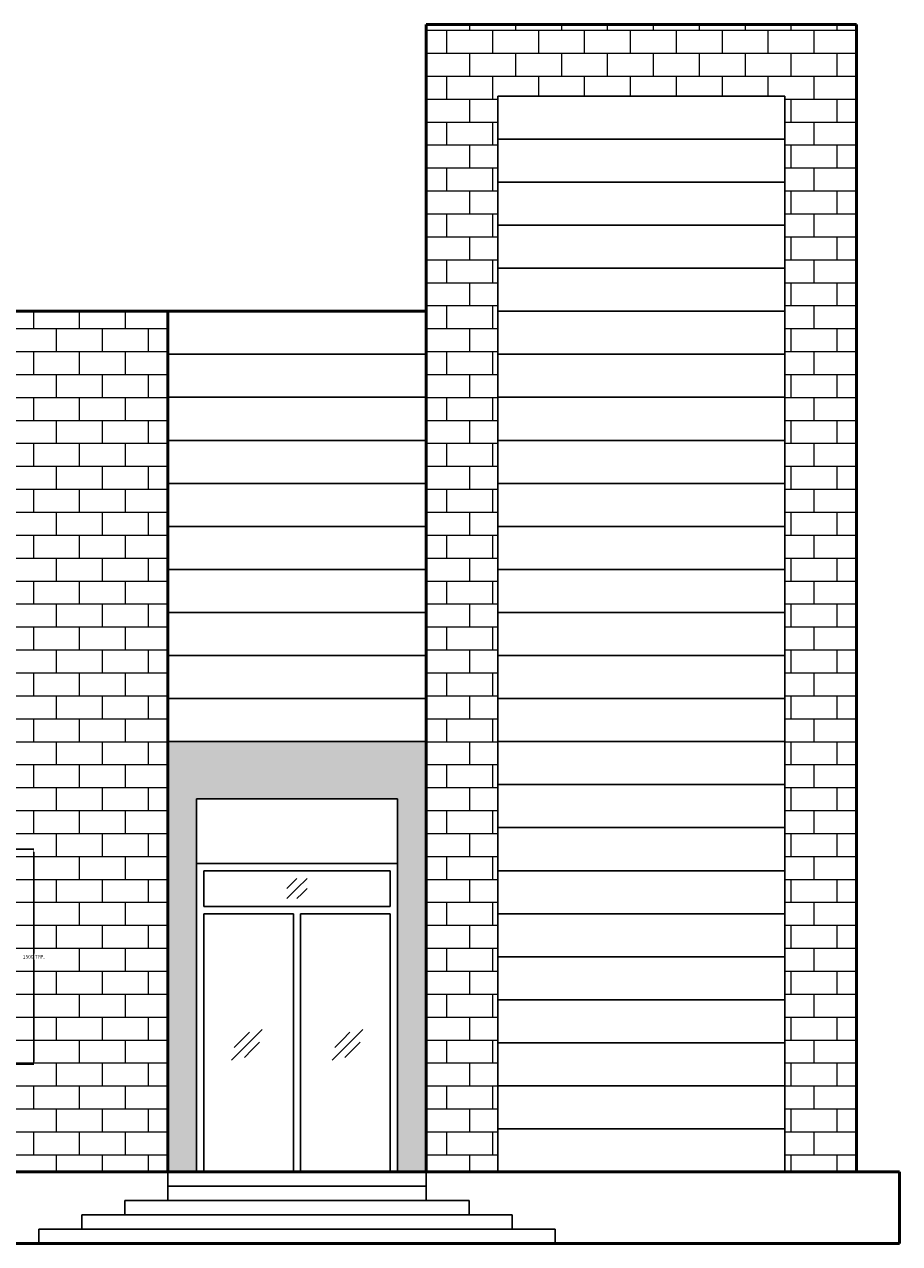
# Model space of a CAD drawing. Units: centimetres. Extents: x 2755 to 12755, y 4821 to 13321.
# Tile 2 of 2: x 6655 to 12755, y 4821 to 13321. Entities that reach past the tile are written whole.
import ezdxf

# ---------------------------------------------------------------- set-up
doc = ezdxf.new("R2010")
doc.units = ezdxf.units.CM
doc.header["$MEASUREMENT"] = 0
for name, color, linetype, lineweight in [('A-ANNO-DIMS', 2, 'Continuous', 18), ('A-DOOR', 3, 'Continuous', 25), ('A-ELEV', 7, 'Continuous', 25), ('A-FLOR-STRS', 7, 'Continuous', 25), ('A-WALL', 7, 'Continuous', 50), ('A-WALL-PATT', 8, 'Continuous', 13)]:
    doc.layers.add(name, color=color, linetype=linetype, lineweight=lineweight)
doc.styles.get("Standard").update_dxf_attribs({"font": 'arial.ttf'})
doc.dimstyles.get("Standard").update_dxf_attribs({"dimtxt": 25, "dimasz": 20, "dimexe": 0.18, "dimexo": 0.0625, "dimgap": 10, "dimtad": 0, "dimtih": 1, "dimtoh": 1, "dimdec": 0, "dimzin": 0, "dimdsep": 46, "dimtxsty": 'Standard', "dimcen": 10, "dimadec": 0, "dimazin": 0, "dimtfac": 1, "dimtdec": 0, "dimtofl": 0, "dimtmove": 0, "dimatfit": 3, "dimfxl": 1, "dimtolj": 1, "dimtzin": 0, "dimarcsym": 0})

# ---------------------------------------------------------------- blocks, each defined once
blk = doc.blocks.new('*U1')
blk.add_line((0, 2000), (0, 0))
blk = doc.blocks.new('*U2')
at = {"layer": 'A-ELEV', "color": 0, "linetype": 'ByBlock', "lineweight": -2, "transparency": 16777216, "rotation": 270}
for p in [(9955.3, 12820.8), (9955.3, 12520.8), (9955.3, 12220.8), (9955.3, 11920.8), (9955.3, 11620.8), (9955.3, 11320.8), (9955.3, 11020.8), (9955.3, 10720.8), (9955.3, 10420.8), (9955.3, 10120.8), (9955.3, 9820.8), (9955.3, 9520.8), (9955.3, 9220.8), (9955.3, 8920.8), (9955.3, 8620.8), (9955.3, 8320.8), (9955.3, 8020.8), (9955.3, 7720.8), (9955.3, 7420.8), (9955.3, 7120.8), (9955.3, 6820.8), (9955.3, 6520.8), (9955.3, 6220.8), (9955.3, 5920.8), (9955.3, 5620.8), (9955.3, 5320.8)]:
    blk.add_blockref('*U1', p, dxfattribs=at)
blk = doc.blocks.new('*D5')
at = {"layer": 'A-ANNO-DIMS', "color": 0, "lineweight": -2, "transparency": 16777216}
for p, q in [((6405.4, 7570.8), (6720.5, 7570.8)), ((6720.3, 7550.8), (6720.3, 6843.6)), ((6720.3, 6090.8), (6720.3, 6798.1)), ((6405.4, 6070.8), (6720.5, 6070.8))]:
    blk.add_line(p, q, dxfattribs=at)
at = {"layer": 'A-ANNO-DIMS', "color": 0, "transparency": 16777216}
for points in [[(6717, 7550.8), (6723.7, 7550.8), (6720.3, 7570.8)], [(6717, 6090.8), (6723.7, 6090.8), (6720.3, 6070.8)]]:
    blk.add_solid(points, dxfattribs=at)
at = {"layer": 'Defpoints', "color": 0, "transparency": 16777216}
for p in [(6405.3, 7570.8), (6720.3, 7570.8), (6405.3, 6070.8)]:
    blk.add_point(p, dxfattribs=at)
at = {"layer": 'A-ANNO-DIMS', "color": 0, "transparency": 16777216, "insert": (6720.3, 6820.8), "char_height": 25, "attachment_point": 5}
blk.add_mtext('\\A1;1500 TYP.', dxfattribs=at)

msp = doc.modelspace()

# ---------------------------------------------------------------- hatches: boundary and pattern name
at = {"layer": 'A-WALL-PATT'}
h = msp.add_hatch(dxfattribs=at)
h.set_pattern_fill('AR-B816', color=256, scale=20)
h.paths.add_polyline_path([(7655.3, 11320.8), (3055.3, 11320.8), (3055.3, 5320.8), (7655.3, 5320.8)])
h.paths.add_polyline_path([(4305.3, 7570.8), (6405.3, 7570.8), (6405.3, 6070.8), (4305.3, 6070.8)], flags=16)
h.paths.add_polyline_path([(4330.3, 7545.8), (6380.3, 7545.8), (6380.3, 6095.8), (4330.3, 6095.8)], flags=0)
h.paths.add_polyline_path([(4305.3, 9070.8), (4305.3, 10570.8), (6405.3, 10570.8), (6405.3, 9070.8)], flags=16)
h.paths.add_polyline_path([(4330.3, 9095.8), (4330.3, 10545.8), (6380.3, 10545.8), (6380.3, 9095.8)], flags=0)
h.paths.add_polyline_path([(9955.3, 12820.8), (11955.3, 12820.8), (11955.3, 5320.8), (12455.3, 5320.8), (12455.3, 13320.8), (9455.3, 13320.8), (9455.3, 11320.8), (9455.3, 5320.8), (9955.3, 5320.8)])
h = msp.add_hatch(dxfattribs=at)
h.set_pattern_fill('EARTH', color=256, scale=200)
h.paths.add_polyline_path([(9455.3, 8320.8), (7655.3, 8320.8), (7655.3, 5320.8), (7855.3, 5320.8), (7855.3, 7920.8), (9255.3, 7920.8), (9255.3, 5320.8), (9455.3, 5320.8)])

# ---------------------------------------------------------------- linework, layer by layer
at = {"layer": 'A-DOOR'}
for p, q in [((7855.3, 7920.8), (9255.3, 7920.8)), ((7855.3, 7920.8), (7855.3, 5320.8)), ((9255.3, 7920.8), (9255.3, 5320.8)), ((7855.3, 7470.8), (9255.3, 7470.8)), ((7905.3, 7420.8), (9205.3, 7420.8)), ((7905.3, 7420.8), (7905.3, 7172)), ((9205.3, 7420.8), (9205.3, 7172)), ((8520, 7331.9), (8484.6, 7296.5)), ((8520, 7331.9), (8555.3, 7367.2)), ((8555.3, 7296.5), (8626, 7367.2)), ((8555.3, 7296.5), (8484.6, 7225.8)), ((8590.7, 7261.2), (8555.3, 7225.8)), ((8590.7, 7261.2), (8626, 7296.5)), ((7905.3, 7172), (9205.3, 7172)), ((7905.3, 7120.8), (8530.3, 7120.8)), ((7905.3, 7120.8), (7905.3, 5320.8)), ((8530.3, 7120.8), (8530.3, 5320.8)), ((8580.3, 7120.8), (8580.3, 5320.8)), ((8580.3, 7120.8), (9205.3, 7120.8)), ((9205.3, 7120.8), (9205.3, 5320.8)), ((8170.6, 6241.9), (8223.6, 6294.9)), ((8206, 6206.5), (8312, 6312.6)), ((8871.7, 6241.9), (8924.7, 6294.9)), ((8907, 6206.5), (9013.1, 6312.6)), ((8206, 6206.5), (8099.9, 6100.4)), ((8170.6, 6241.9), (8117.6, 6188.8)), ((8241.3, 6171.2), (8294.3, 6224.2)), ((8907, 6206.5), (8801, 6100.4)), ((8871.7, 6241.9), (8818.7, 6188.8)), ((8942.4, 6171.2), (8995.4, 6224.2)), ((8241.3, 6171.2), (8188.3, 6118.1)), ((8942.4, 6171.2), (8889.4, 6118.1))]:
    msp.add_line(p, q, dxfattribs=at)
at = {"layer": 'A-ELEV'}
for p, q in [((9955.3, 12820.8), (9955.3, 5320.8)), ((11955.3, 5320.8), (11955.3, 12820.8)), ((7655.3, 11020.8), (9455.3, 11020.8)), ((7655.3, 10720.8), (9455.3, 10720.8)), ((7655.3, 10420.8), (9455.3, 10420.8)), ((7655.3, 10120.8), (9455.3, 10120.8)), ((7655.3, 9820.8), (9455.3, 9820.8)), ((7655.3, 9520.8), (9455.3, 9520.8)), ((7655.3, 9220.8), (9455.3, 9220.8)), ((7655.3, 8920.8), (9455.3, 8920.8)), ((7655.3, 8620.8), (9455.3, 8620.8)), ((7655.3, 8320.8), (9455.3, 8320.8))]:
    msp.add_line(p, q, dxfattribs=at)
at = {"layer": 'A-FLOR-STRS'}
for p, q in [((7655.3, 5320.8), (7655.3, 5120.8)), ((9455.3, 5320.8), (9455.3, 5120.8)), ((7655.3, 5220.8), (9455.3, 5220.8)), ((7655.3, 5120.8), (7355.3, 5120.8)), ((7355.3, 5120.8), (7355.3, 5020.8)), ((7655.3, 5120.8), (9455.3, 5120.8)), ((9455.3, 5120.8), (9755.3, 5120.8)), ((9755.3, 5120.8), (9755.3, 5020.8)), ((7355.3, 5020.8), (7055.3, 5020.8)), ((7055.3, 5020.8), (7055.3, 4920.8)), ((9755.3, 5020.8), (7355.3, 5020.8)), ((9755.3, 5020.8), (10055.3, 5020.8)), ((10055.3, 5020.8), (10055.3, 4920.8)), ((7055.3, 4920.8), (6755.3, 4920.8)), ((6755.3, 4920.8), (6755.3, 4820.8)), ((7055.3, 4920.8), (10055.3, 4920.8)), ((10055.3, 4920.8), (10355.3, 4920.8)), ((10355.3, 4920.8), (10355.3, 4820.8)), ((6755.3, 4820.8), (10355.3, 4820.8))]:
    msp.add_line(p, q, dxfattribs=at)
at = {"layer": 'A-WALL'}
for p, q in [((12455.3, 13320.8), (9455.3, 13320.8)), ((9455.3, 13320.8), (9455.3, 11320.8)), ((12455.3, 5320.8), (12455.3, 13320.8)), ((9455.3, 11320.8), (3055.3, 11320.8)), ((7655.3, 11320.8), (7655.3, 5320.8)), ((9455.3, 11320.8), (9455.3, 5320.8)), ((12755.3, 5320.8), (2755.3, 5320.8)), ((12755.3, 4820.8), (12755.3, 5320.8)), ((2755.3, 4820.8), (12755.3, 4820.8))]:
    msp.add_line(p, q, dxfattribs=at)

# ---------------------------------------------------------------- block references
at = {"layer": 'A-ELEV'}
msp.add_blockref('*U2', (0, 0), dxfattribs=at)

# ---------------------------------------------------------------- dimensions: what is measured, and where the dimension line sits
at = {"layer": 'A-ANNO-DIMS'}
dim = msp.add_linear_dim(base=(6720.3, 7570.8), p1=(6405.3, 6070.8), p2=(6405.3, 7570.8), angle=90, text='<> TYP.', dimstyle='Standard', override={"dimdec": 0, "dimlfac": 1, "dimrnd": 0, "dimzin": 0, "dimdsep": 46, "dimlunit": 2}, dxfattribs=at)
dim.commit()
dim.dimension.update_dxf_attribs({"geometry": '*D5', "text_midpoint": (6720.3, 6820.8)})

doc.saveas('drawing.dxf')
